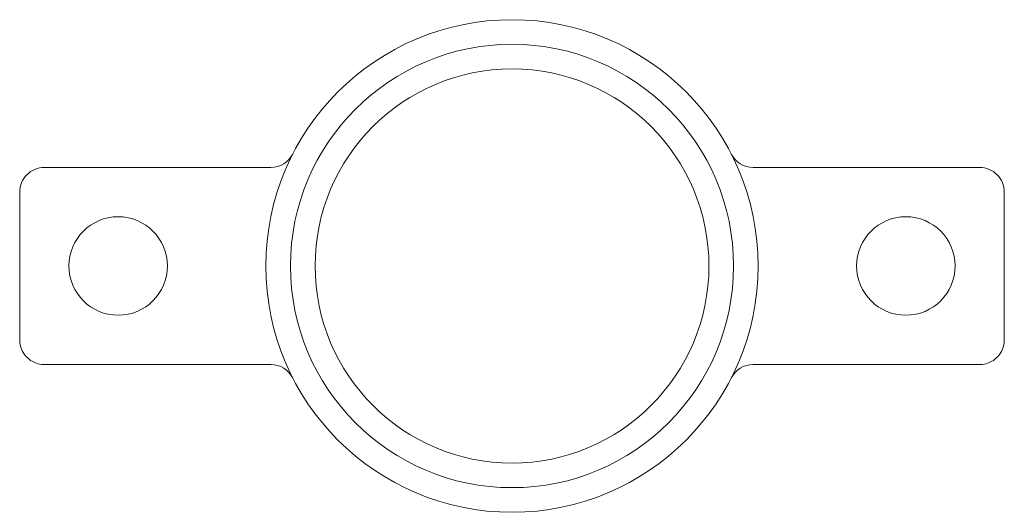
# Model space of a CAD drawing. Units: millimetres. Extents: x 3830 to 4030, y 1968 to 2068.
import ezdxf

# ---------------------------------------------------------------- set-up
doc = ezdxf.new("R2010")
doc.units = ezdxf.units.MM
doc.layers.add('M-CONS', color=8, linetype='Continuous', lineweight=18)

msp = doc.modelspace()

# ---------------------------------------------------------------- linework, layer by layer
at = {"layer": 'M-CONS'}
msp.add_line((3829.93, 2018), (3829.93, 2033), dxfattribs=at)
for points in [[(3885.39, 2040.73, -0.281861), (3880.94, 2038), (3834.93, 2038, 0.414214), (3829.93, 2033), (3829.93, 2003, 0.414214), (3834.93, 1998), (3880.94, 1998, -0.281861), (3885.39, 1995.27)], [(3974.46, 1995.27, -0.281861), (3978.92, 1998), (4024.93, 1998, 0.414214), (4029.93, 2003), (4029.93, 2033, 0.414214), (4024.93, 2038), (3978.92, 2038, -0.281861), (3974.46, 2040.73)]]:
    msp.add_lwpolyline(points, format="xyb", dxfattribs=at)
for centre, radius in [((3929.93, 2018), 50), ((3929.93, 2018), 45), ((3929.93, 2018), 40), ((3849.93, 2018), 10), ((4009.93, 2018), 10)]:
    msp.add_circle(centre, radius, dxfattribs=at)

doc.saveas('drawing.dxf')
